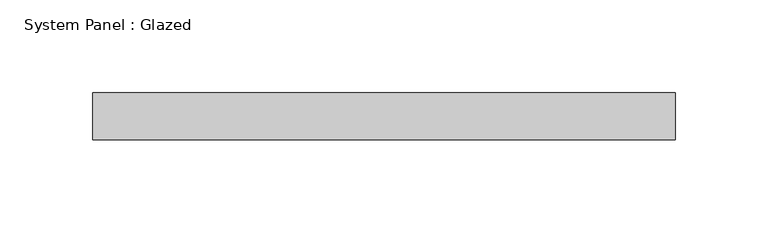
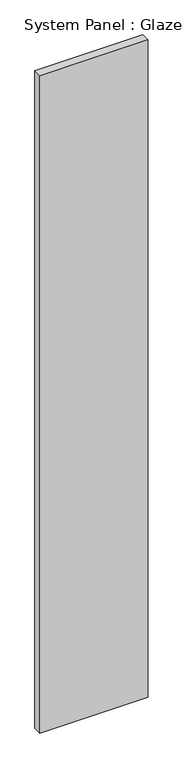
"""IFC4 building model written with IfcOpenShell, lengths in millimetres: plate geometry, System Panel : Glazed."""

from ifc_helpers import new_model, si_unit, origin, origin_with_axes, place, context, project, spatial, polyline, outline, extrude, source, transform, mapped, element, save


def system_panel_glazed_11fb153e(model_context):
    return source(origin(), model_context, "Body", "SweptSolid", [
        extrude(outline(polyline([(157.3561662, 19.05), (-157.3561662, 19.05), (-157.3561662, 44.45), (157.3561662, 44.45), (157.3561662, 19.05)])), origin_with_axes(), (0.0, 0.0, 1.0), 2032.0),
    ])


if __name__ == "__main__":
    model = new_model("IFC4")
    model_context = context("Model", 3, world=origin())
    ifc_project = project(units=[si_unit("LENGTHUNIT", "METRE", prefix="MILLI")], contexts=[model_context])
    site = spatial("IfcSite", under=ifc_project)
    building = spatial("IfcBuilding", under=site)
    placement = place(None, origin())
    system_panel_glazed_shape = system_panel_glazed_11fb153e(model_context)
    element("IfcPlate", 1, ObjectType="System Panel : Glazed", at=placement, inside=building, context=model_context, shape_type="MappedRepresentation", body=[
        mapped(system_panel_glazed_shape, transform((0.0, 0.0, 0.0), x_axis=(1.0, 0.0, 0.0), y_axis=(0.0, 1.0, 0.0), z_axis=(0.0, 0.0, 1.0))),
    ])
    save(model, "model.ifc")

# Revit data of these elements
# Type "System Panel : Glazed"
#   Construction Type Id = "GSP4R"
#   Analytic Construction = "1/8 in Pilkington single glazing"
#   Visual Light Transmittance = 0.9
#   Solar Heat Gain Coefficient = 0.86
#   Heat Transfer Coefficient (U) = 1.18115 BTU/(h·ft²·°F)
# Element 1 (IfcPlate, "System Panel : Glazed")
#   Materials on its faces: "Glass"
# Materials
#   "Glass": class "Glass", colour RGB 0 128 192, transparency 0.75, Description = "Soda Lime Glass", Cost = 0
